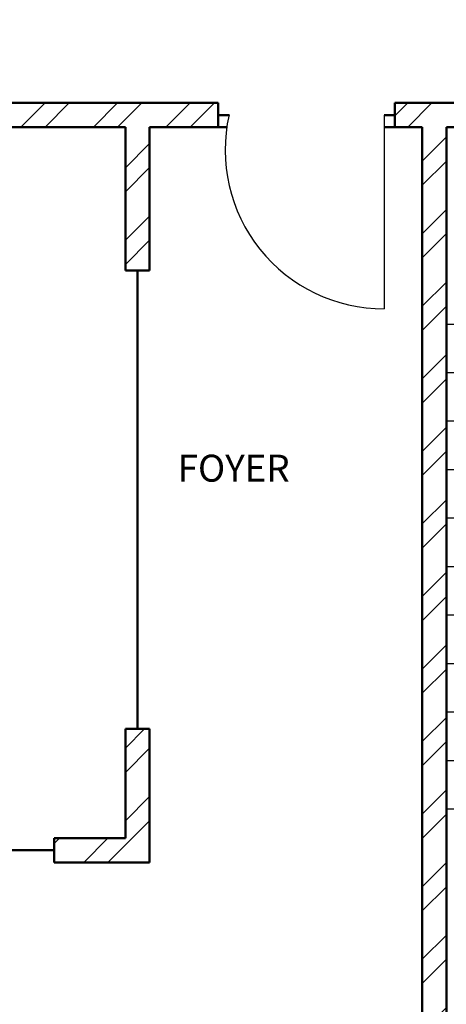
# Model space of a CAD drawing. Units: inches. Extents: x 1901 to 2863, y 888 to 2433.
# Tile 20 of 91: x 2264 to 2343, y 1549 to 1732. Entities that reach past the tile are written whole.
import ezdxf

# ---------------------------------------------------------------- set-up
doc = ezdxf.new("R2010")
doc.units = ezdxf.units.IN
for name, color, linetype, lineweight in [('A-AREA-IDEN', 7, 'Continuous', 18), ('A-DOOR', 4, 'Continuous', 25), ('A-FLOR-STRS', 2, 'Continuous', 25), ('A-WALL', 7, 'Continuous', 50), ('A-WALL-PATT', 8, 'Continuous', 13)]:
    doc.layers.add(name, color=color, linetype=linetype, lineweight=lineweight)
doc.styles.get("Standard").update_dxf_attribs({"font": 'arial.ttf'})

msp = doc.modelspace()

# ---------------------------------------------------------------- hatches: boundary and pattern name
at = {"layer": 'A-WALL-PATT'}
h = msp.add_hatch(dxfattribs=at)
h.set_pattern_fill('ANSI32', color=256)
h.paths.add_polyline_path([(2192.5, 2274.13), (2141.26, 2274.13), (2141.26, 2269.63), (2192.5, 2269.63)])
h.paths.add_polyline_path([(2259.93, 2274.13), (2216.5, 2274.13), (2216.5, 2269.63), (2255.43, 2269.63), (2255.43, 2214.63), (2250.81, 2214.63), (2250.81, 2210.13), (2259.93, 2210.13), (2259.93, 2215.13), (2271.76, 2215.13), (2271.76, 2217.38), (2271.76, 2219.63), (2259.93, 2219.63)])
h.paths.add_polyline_path([(2171.43, 2269.63), (2166.93, 2269.63), (2166.93, 2219.63), (2121.24, 2219.63), (2121.24, 2215.13), (2166.93, 2215.13), (2166.93, 2083.13), (2161.81, 2083.13), (2161.81, 2078.63), (2171.43, 2078.63), (2177, 2078.63), (2177, 2080.88), (2177, 2083.13), (2171.43, 2083.13), (2171.43, 2210.13), (2230.91, 2210.13), (2230.91, 2212.38), (2230.91, 2214.63), (2171.43, 2214.63)])
h.paths.add_polyline_path([(2117.26, 2274.13), (2089.43, 2274.13), (2089.43, 2219.63), (2081.14, 2219.63), (2081.14, 2215.13), (2089.43, 2215.13), (2098, 2215.13), (2098, 2217.38), (2098, 2219.63), (2093.93, 2219.63), (2093.93, 2269.63), (2117.26, 2269.63), (2117.26, 2271.88)])
h.paths.add_polyline_path([(2343.43, 2219.63), (2329.29, 2219.63), (2329.29, 2215.13), (2338.93, 2215.13), (2338.93, 2184.74), (2343.43, 2184.74)])
h.paths.add_polyline_path([(2338.93, 2083.13), (2329.29, 2083.13), (2208.97, 2083.13), (2208.97, 2078.63), (2338.93, 2078.63)])
h.paths.add_polyline_path([(2343.43, 2136.74), (2338.93, 2136.74), (2338.93, 1872.63), (2343.43, 1872.63)])
h.paths.add_polyline_path([(2343.43, 1863.63), (2397.68, 1863.63), (2397.68, 1821.63), (2384.14, 1821.63), (2384.14, 1812.63), (2418.33, 1812.63), (2418.33, 1817.13), (2418.33, 1821.63), (2406.68, 1821.63), (2406.68, 1863.63), (2459.5, 1863.63), (2459.5, 1821.63), (2447.14, 1821.63), (2447.14, 1812.63), (2459.5, 1812.63), (2468.5, 1812.63), (2468.5, 1872.63), (2394.43, 1872.63), (2334.43, 1872.63), (2334.43, 1812.63), (2343.43, 1812.63), (2353.25, 1812.63), (2353.25, 1821.63), (2343.43, 1821.63)])
h.paths.add_polyline_path([(2510.01, 1872.63), (2468.5, 1872.63), (2468.5, 1868.13), (2510.01, 1868.13)])
h.paths.add_polyline_path([(2514.01, 1817.13), (2468.5, 1817.13), (2468.5, 1812.63), (2482.11, 1812.63), (2482.11, 1800.61), (2486.61, 1800.61), (2486.61, 1812.63), (2514.01, 1812.63)])
h.paths.add_polyline_path([(2299.25, 1814.88), (2299.25, 1817.13), (2295.93, 1817.13), (2295.93, 1854.17), (2293.68, 1854.17), (2291.43, 1854.17), (2291.43, 1817.13), (2266.11, 1817.13), (2266.11, 1812.63), (2299.25, 1812.63)])
h.paths.add_polyline_path([(2218.11, 1817.13), (2206.46, 1817.13), (2171.43, 1817.13), (2171.43, 1949.13), (2190.1, 1949.13), (2190.1, 1953.63), (2163.47, 1953.63), (2163.47, 1949.13), (2166.93, 1949.13), (2166.93, 1817.13), (2114.3, 1817.13), (2114.3, 1812.63), (2218.11, 1812.63)])
h.paths.add_polyline_path([(2029.43, 1970.92), (2024.93, 1970.92), (2024.93, 1912.72), (2029.43, 1912.72)])
h.paths.add_polyline_path([(2132.3, 1953.63), (2113.93, 1953.63), (2113.93, 1975.89), (2111.68, 1975.89), (2109.43, 1975.89), (2109.43, 1953.63), (2029.43, 1953.63), (2029.43, 1949.13), (2132.3, 1949.13)])
h.paths.add_polyline_path([(2029.43, 1853.61), (2029.31, 1853.61), (2029.31, 1853.61), (2029.43, 1853.61), (2029.43, 1864.72), (2024.93, 1864.72), (2024.93, 1812.63), (2066.3, 1812.63), (2066.3, 1814.88), (2066.3, 1817.13), (2029.43, 1817.13)])
h.paths.add_polyline_path([(2122.93, 2010.09), (2120.68, 2010.09), (2118.43, 2010.09), (2118.43, 2006.13), (2029.43, 2006.13), (2029.43, 2001.63), (2109.43, 2001.63), (2109.43, 1998.04), (2113.93, 1998.04), (2113.93, 2001.63), (2122.93, 2001.63)])
h.paths.add_polyline_path([(2029.43, 2031.38), (2024.93, 2031.38), (2024.93, 1994.92), (2027.18, 1994.92), (2029.43, 1994.92)])
h.paths.add_polyline_path([(2029.43, 2136.74), (2024.93, 2136.74), (2024.93, 2067.38), (2027.18, 2067.38), (2029.43, 2067.38)])
h.paths.add_polyline_path([(2125.62, 2083.13), (2029.43, 2083.13), (2029.43, 2078.63), (2118.43, 2078.63), (2118.43, 2030.71), (2122.93, 2030.71), (2122.93, 2078.63), (2125.62, 2078.63)])
h.paths.add_polyline_path([(2029.43, 2215.13), (2040.47, 2215.13), (2040.47, 2217.38), (2040.47, 2219.63), (2024.93, 2219.63), (2024.93, 2184.74), (2029.43, 2184.74), (2029.43, 2187.78)])
h.paths.add_polyline_path([(2686.43, 2274.13), (2659.28, 2274.13), (2659.28, 2269.63), (2681.93, 2269.63), (2681.93, 2219.63), (2676.82, 2219.63), (2676.82, 2215.13), (2681.93, 2215.13), (2697.01, 2215.13), (2697.01, 2217.38), (2697.01, 2219.63), (2686.43, 2219.63)])
h.paths.add_polyline_path([(2609.93, 2269.63), (2635.28, 2269.63), (2635.28, 2274.13), (2571.43, 2274.13), (2571.43, 2269.63), (2605.43, 2269.63), (2605.43, 2214.63), (2549.1, 2214.63), (2549.1, 2210.13), (2605.43, 2210.13), (2605.43, 2083.13), (2601.01, 2083.13), (2601.01, 2080.88), (2601.01, 2078.63), (2609.93, 2078.63), (2616.16, 2078.63), (2616.16, 2080.88), (2616.16, 2083.13), (2609.93, 2083.13), (2609.93, 2215.13), (2651.46, 2215.13), (2651.46, 2217.38), (2651.46, 2219.63), (2609.93, 2219.63)])
h.paths.add_polyline_path([(2521.43, 2269.63), (2547.43, 2269.63), (2547.43, 2271.88), (2547.43, 2274.13), (2516.93, 2274.13), (2516.93, 2219.63), (2506.41, 2219.63), (2506.41, 2215.13), (2516.93, 2215.13), (2516.93, 2210.13), (2525.4, 2210.13), (2525.4, 2212.38), (2525.4, 2214.63), (2521.43, 2214.63)])
h.paths.add_polyline_path([(2456.01, 2219.63), (2439.43, 2219.63), (2439.43, 2187.89), (2443.93, 2187.89), (2443.93, 2215.13), (2456.01, 2215.13)])
h.paths.add_polyline_path([(2752.93, 2219.63), (2739.48, 2219.63), (2739.48, 2215.13), (2748.43, 2215.13), (2748.43, 2187.89), (2752.93, 2187.89)])
h.paths.add_polyline_path([(2752.93, 2139.89), (2748.43, 2139.89), (2748.43, 2083.13), (2648.42, 2083.13), (2648.42, 2078.63), (2654.93, 2078.63), (2654.93, 2039.44), (2659.43, 2039.44), (2659.43, 2078.63), (2748.43, 2078.63), (2748.43, 2063.43), (2752.93, 2063.43)])
h.paths.add_polyline_path([(2752.93, 2010.63), (2659.43, 2010.63), (2659.43, 2015.65), (2654.93, 2015.65), (2654.93, 2010.63), (2605.43, 2010.63), (2605.43, 1920.97), (2609.93, 1920.97), (2609.93, 2006.13), (2748.43, 2006.13), (2748.43, 1982.47), (2752.93, 1982.47)])
h.paths.add_polyline_path([(2752.93, 2027.43), (2748.43, 2027.43), (2748.43, 2010.63), (2752.93, 2010.63)])
h.paths.add_polyline_path([(2748.43, 1886.13), (2609.93, 1886.13), (2609.93, 1889.72), (2605.43, 1889.72), (2605.43, 1861.26), (2609.93, 1861.26), (2609.93, 1881.63), (2748.43, 1881.63)])
h.paths.add_polyline_path([(2456.86, 2228.83), (2498.4, 2228.83), (2498.4, 2247.49), (2456.86, 2247.49)], flags=9)
h.paths.add_polyline_path([(2038.6, 2237.42), (2080.17, 2237.42), (2080.17, 2256.08), (2038.6, 2256.08)], flags=9)
h.paths.add_polyline_path([(2292.01, 1062.39), (2539.93, 1062.39), (2539.93, 1099.49), (2292.01, 1099.49)], flags=9)
h.paths.add_polyline_path([(2424.91, 1832.25), (2448.51, 1832.25), (2448.51, 1846.68), (2424.91, 1846.68)], flags=25)
h.paths.add_polyline_path([(2359.08, 1832.25), (2382.68, 1832.25), (2382.68, 1846.68), (2359.08, 1846.68)], flags=25)
h.paths.add_polyline_path([(2352.9, 1684.8), (2367.54, 1684.8), (2367.54, 1697.17), (2352.9, 1697.17)], flags=9)
h.paths.add_polyline_path([(2079.29, 1755.83), (2169.02, 1755.83), (2169.02, 1774.37), (2079.29, 1774.37)], flags=9)
h.paths.add_polyline_path([(2404.09, 1373.86), (2404.09, 1463.59), (2385.54, 1463.59), (2385.54, 1373.86)], flags=9)
h.paths.add_polyline_path([(2268.09, 2236.37), (2309.64, 2236.37), (2309.64, 2255.03), (2268.09, 2255.03)], flags=9)
h.paths.add_polyline_path([(2575.96, 1700.95), (2665.7, 1700.95), (2665.7, 1719.5), (2575.96, 1719.5)], flags=9)
h.paths.add_polyline_path([(2302.96, 1878.47), (2329.52, 1878.47), (2329.52, 1888.78), (2302.96, 1888.78)], flags=9)
h.paths.add_polyline_path([(2097.42, 2240.58), (2126.57, 2240.58), (2126.57, 2259.23), (2097.42, 2259.23)], flags=9)
h.paths.add_polyline_path([(2208.72, 2246.12), (2237.88, 2246.12), (2237.88, 2264.78), (2208.72, 2264.78)], flags=9)
h.paths.add_polyline_path([(2038.15, 1925.96), (2076.99, 1925.96), (2076.99, 1944.62), (2038.15, 1944.62)], flags=9)
h.paths.add_polyline_path([(2239.14, 1926.67), (2288.46, 1926.67), (2288.46, 1945.33), (2239.14, 1945.33)], flags=9)
h.paths.add_polyline_path([(2175.43, 2007.33), (2212.36, 2007.33), (2212.36, 2025.99), (2175.43, 2025.99)], flags=9)
h.paths.add_polyline_path([(2225.03, 2091.79), (2263.87, 2091.79), (2263.87, 2110.45), (2225.03, 2110.45)], flags=9)
h.paths.add_polyline_path([(2035.4, 2098.48), (2074.24, 2098.48), (2074.24, 2117.14), (2035.4, 2117.14)], flags=9)
h.paths.add_polyline_path([(2050.1, 2029.21), (2083.26, 2029.21), (2083.26, 2047.87), (2050.1, 2047.87)], flags=9)
h.paths.add_polyline_path([(2069.68, 1956.72), (2098.83, 1956.72), (2098.83, 1975.38), (2069.68, 1975.38)], flags=25)
h.paths.add_polyline_path([(2328.62, 1753.34), (2361.66, 1753.34), (2361.66, 1771.99), (2328.62, 1771.99)], flags=9)
h.paths.add_polyline_path([(2395.16, 2060.89), (2395.16, 2140.65), (2378.68, 2140.65), (2378.68, 2060.89)], flags=9)
h.paths.add_polyline_path([(2463.73, 2059.02), (2492.89, 2059.02), (2492.89, 2077.68), (2463.73, 2077.68)], flags=9)
h.paths.add_polyline_path([(2458.03, 2181.54), (2496.87, 2181.54), (2496.87, 2200.19), (2458.03, 2200.19)], flags=9)
h.paths.add_polyline_path([(2527.58, 2243.07), (2556.73, 2243.07), (2556.73, 2261.73), (2527.58, 2261.73)], flags=9)
h.paths.add_polyline_path([(2694.46, 2232.77), (2736.03, 2232.77), (2736.03, 2251.42), (2694.46, 2251.42)], flags=9)
h.paths.add_polyline_path([(2637.82, 2249.22), (2666.98, 2249.22), (2666.98, 2267.88), (2637.82, 2267.88)], flags=9)
h.paths.add_polyline_path([(2623.69, 2183.54), (2662.53, 2183.54), (2662.53, 2202.2), (2623.69, 2202.2)], flags=9)
h.paths.add_polyline_path([(2691.97, 2021.5), (2725.12, 2021.5), (2725.12, 2040.16), (2691.97, 2040.16)], flags=9)
h.paths.add_polyline_path([(2621.04, 1975.91), (2662.34, 1975.91), (2662.34, 1994.57), (2621.04, 1994.57)], flags=25)
h.paths.add_polyline_path([(2479.03, 1927.62), (2519.84, 1927.62), (2519.84, 1946.28), (2479.03, 1946.28)], flags=9)
h.paths.add_polyline_path([(2670.94, 1849.08), (2716.01, 1849.08), (2716.01, 1867.73), (2670.94, 1867.73)], flags=9)
h.paths.add_polyline_path([(2523.61, 1782.96), (2550.17, 1782.96), (2550.17, 1793.26), (2523.61, 1793.26)], flags=9)
h.paths.add_polyline_path([(2450.84, 1207.33), (2492.39, 1207.33), (2492.39, 1225.99), (2450.84, 1225.99)], flags=9)
h.paths.add_polyline_path([(2527.75, 1203.84), (2556.91, 1203.84), (2556.91, 1222.5), (2527.75, 1222.5)], flags=9)
h.paths.add_polyline_path([(2639.11, 1207.2), (2668.27, 1207.2), (2668.27, 1225.86), (2639.11, 1225.86)], flags=9)
h.paths.add_polyline_path([(2692.59, 1218.97), (2734.17, 1218.97), (2734.17, 1237.62), (2692.59, 1237.62)], flags=9)
h.paths.add_polyline_path([(2669.27, 1366.33), (2708.11, 1366.33), (2708.11, 1384.99), (2669.27, 1384.99)], flags=9)
h.paths.add_polyline_path([(2463.31, 1358.03), (2502.15, 1358.03), (2502.15, 1376.69), (2463.31, 1376.69)], flags=9)
h.paths.add_polyline_path([(2494.72, 1449.96), (2531.65, 1449.96), (2531.65, 1468.62), (2494.72, 1468.62)], flags=9)
h.paths.add_polyline_path([(2675.57, 1422.16), (2708.72, 1422.16), (2708.72, 1440.81), (2675.57, 1440.81)], flags=9)
h.paths.add_polyline_path([(2685.63, 1493.89), (2714.79, 1493.89), (2714.79, 1512.55), (2685.63, 1512.55)], flags=9)
h.paths.add_polyline_path([(2686.8, 1529.91), (2725.65, 1529.91), (2725.65, 1548.57), (2686.8, 1548.57)], flags=9)
h.paths.add_polyline_path([(2503.65, 1537.99), (2552.97, 1537.99), (2552.97, 1556.65), (2503.65, 1556.65)], flags=9)
h.paths.add_polyline_path([(2291.71, 1643.5), (2318.28, 1643.5), (2318.28, 1653.81), (2291.71, 1653.81)], flags=9)
h.paths.add_polyline_path([(2450.63, 1610.52), (2477.19, 1610.52), (2477.19, 1620.82), (2450.63, 1620.82)], flags=9)
h.paths.add_polyline_path([(2359.99, 1551.81), (2422.25, 1551.81), (2422.25, 1562.12), (2359.99, 1562.12)], flags=9)
h.paths.add_polyline_path([(2280.11, 1249.01), (2321.65, 1249.01), (2321.65, 1267.66), (2280.11, 1267.66)], flags=9)
h.paths.add_polyline_path([(2164.06, 1274.23), (2193.22, 1274.23), (2193.22, 1292.89), (2164.06, 1292.89)], flags=9)
h.paths.add_polyline_path([(2118.21, 1277.69), (2151.25, 1277.69), (2151.25, 1296.35), (2118.21, 1296.35)], flags=9)
h.paths.add_polyline_path([(2031.95, 1268.53), (2073.52, 1268.53), (2073.52, 1287.19), (2031.95, 1287.19)], flags=9)
h.paths.add_polyline_path([(2050.2, 1409.08), (2089.04, 1409.08), (2089.04, 1427.74), (2050.2, 1427.74)], flags=9)
h.paths.add_polyline_path([(2243.74, 1421.03), (2282.58, 1421.03), (2282.58, 1439.69), (2243.74, 1439.69)], flags=9)
h.paths.add_polyline_path([(2190.75, 1509.77), (2231.56, 1509.77), (2231.56, 1528.43), (2190.75, 1528.43)], flags=9)
h.paths.add_polyline_path([(2058.39, 1475.42), (2091.55, 1475.42), (2091.55, 1494.07), (2058.39, 1494.07)], flags=9)
h.paths.add_polyline_path([(2062.45, 1553.09), (2091.6, 1553.09), (2091.6, 1571.75), (2062.45, 1571.75)], flags=9)
h.paths.add_polyline_path([(2219.52, 1590.37), (2266.15, 1590.37), (2266.15, 1609.02), (2219.52, 1609.02)], flags=9)
h.paths.add_polyline_path([(2041.07, 1584.19), (2079.91, 1584.19), (2079.91, 1602.85), (2041.07, 1602.85)], flags=9)
h = msp.add_hatch(dxfattribs=at)
h.set_pattern_fill('ANSI32', color=256)
h.paths.add_polyline_path([(2443.93, 2139.89), (2439.43, 2139.89), (2439.43, 2069.35), (2441.68, 2069.35), (2443.93, 2069.35), (2443.93, 2078.63), (2521.93, 2078.63), (2521.93, 2075.07), (2524.18, 2075.07), (2526.43, 2075.07), (2526.43, 2078.63), (2571.75, 2078.63), (2571.75, 2080.88), (2571.75, 2083.13), (2443.93, 2083.13)])
h.paths.add_polyline_path([(2526.43, 2054.63), (2524.18, 2054.63), (2521.93, 2054.63), (2521.93, 2030.63), (2443.93, 2030.63), (2443.93, 2045.35), (2439.43, 2045.35), (2439.43, 1983.87), (2443.93, 1983.87), (2443.93, 2026.13), (2521.93, 2026.13), (2526.43, 2026.13)])
h.paths.add_polyline_path([(2443.93, 1923.87), (2439.43, 1923.87), (2439.43, 1872.63), (2443.93, 1872.63)])
h.paths.add_polyline_path([(2636.23, 1766.13), (2609.93, 1766.13), (2609.93, 1779.79), (2605.43, 1779.79), (2605.43, 1766.13), (2486.61, 1766.13), (2486.61, 1770.67), (2482.11, 1770.67), (2482.11, 1766.13), (2482.11, 1761.63), (2636.23, 1761.63), (2636.23, 1763.88)])
h.paths.add_polyline_path([(2519.54, 1663.38), (2519.54, 1665.63), (2494.93, 1665.63), (2481.83, 1665.63), (2481.83, 1663.38), (2481.83, 1661.13), (2490.43, 1661.13), (2490.43, 1640.16), (2494.93, 1640.16), (2494.93, 1661.13), (2519.54, 1661.13)])
h.paths.add_polyline_path([(2443.93, 1712.13), (2443.93, 1716.63), (2414.46, 1716.63), (2414.46, 1712.13), (2439.43, 1712.13), (2439.43, 1545.51), (2443.93, 1545.51), (2443.93, 1661.13), (2448.47, 1661.13), (2448.47, 1665.63), (2443.93, 1665.63)])
h.paths.add_polyline_path([(2343.43, 1712.13), (2365.52, 1712.13), (2365.52, 1714.38), (2365.52, 1716.63), (2333.87, 1716.63), (2333.87, 1714.38), (2333.87, 1712.13), (2338.93, 1712.13), (2338.93, 1575.63), (2338.93, 1545.51), (2343.43, 1545.51), (2343.43, 1547.51), (2343.43, 1580.13)])
h.paths.add_polyline_path([(2752.93, 1665.63), (2579.54, 1665.63), (2579.54, 1661.13), (2615.93, 1661.13), (2615.93, 1529.13), (2598.93, 1529.13), (2598.93, 1524.63), (2623.13, 1524.63), (2623.13, 1526.88), (2623.13, 1529.13), (2620.43, 1529.13), (2620.43, 1661.13), (2748.43, 1661.13), (2748.43, 1633.5), (2752.93, 1633.5)])
h.paths.add_polyline_path([(2752.93, 1419.93), (2748.43, 1419.93), (2748.43, 1400.13), (2659.43, 1400.13), (2659.43, 1444.33), (2657.18, 1444.33), (2654.93, 1444.33), (2654.93, 1400.13), (2643.65, 1400.13), (2643.65, 1395.63), (2748.43, 1395.63), (2748.43, 1364.04), (2752.93, 1364.04)])
h.paths.add_polyline_path([(2752.93, 1492.88), (2748.43, 1492.88), (2748.43, 1476.63), (2667.43, 1476.63), (2667.43, 1479.71), (2665.18, 1479.71), (2662.93, 1479.71), (2662.93, 1476.63), (2654.93, 1476.63), (2654.93, 1469.54), (2659.43, 1469.54), (2659.43, 1472.13), (2748.43, 1472.13), (2748.43, 1455.93), (2752.93, 1455.93)])
h.paths.add_polyline_path([(2752.93, 1304.04), (2748.43, 1304.04), (2748.43, 1263.63), (2738.66, 1263.63), (2738.66, 1259.13), (2752.93, 1259.13)])
h.paths.add_polyline_path([(2685.93, 1259.13), (2695.49, 1259.13), (2695.49, 1261.38), (2695.49, 1263.63), (2677.84, 1263.63), (2677.84, 1261.38), (2677.84, 1259.13), (2681.43, 1259.13), (2681.43, 1203.63), (2653.28, 1203.63), (2653.28, 1199.13), (2685.93, 1199.13), (2685.93, 1203.63)])
h.paths.add_polyline_path([(2609.43, 1395.63), (2611.85, 1395.63), (2611.85, 1400.13), (2598.89, 1400.13), (2598.89, 1397.88), (2598.89, 1395.63), (2604.93, 1395.63), (2604.93, 1268.13), (2554.73, 1268.13), (2554.73, 1265.88), (2554.73, 1263.63), (2604.93, 1263.63), (2604.93, 1203.63), (2571.31, 1203.63), (2571.31, 1199.13), (2604.93, 1199.13), (2629.28, 1199.13), (2629.28, 1201.38), (2629.28, 1203.63), (2609.43, 1203.63), (2609.43, 1258.63), (2609.43, 1259.13), (2654.8, 1259.13), (2654.8, 1263.63), (2609.43, 1263.63)])
h.paths.add_polyline_path([(2443.93, 1304.04), (2439.43, 1304.04), (2439.43, 1259.13), (2443.93, 1259.13), (2456.16, 1259.13), (2456.16, 1261.38), (2456.16, 1263.63), (2443.93, 1263.63)])
h.paths.add_polyline_path([(2525.43, 1263.63), (2531.78, 1263.63), (2531.78, 1268.13), (2520.93, 1268.13), (2520.93, 1263.63), (2511.41, 1263.63), (2511.41, 1259.13), (2520.93, 1259.13), (2520.93, 1199.13), (2547.31, 1199.13), (2547.31, 1201.38), (2547.31, 1203.63), (2525.43, 1203.63)])
h.paths.add_polyline_path([(2443.93, 1434.84), (2439.43, 1434.84), (2439.43, 1364.04), (2441.68, 1364.04), (2443.93, 1364.04)])
h.paths.add_polyline_path([(2567.13, 1400.13), (2443.93, 1400.13), (2443.93, 1395.63), (2567.13, 1395.63)])
h.paths.add_polyline_path([(2443.93, 1545.51), (2439.43, 1545.51), (2439.43, 1494.84), (2443.93, 1494.84)])
h.paths.add_polyline_path([(2494.93, 1553.35), (2492.68, 1553.35), (2490.43, 1553.35), (2490.43, 1524.63), (2494.93, 1524.63), (2525.94, 1524.63), (2525.94, 1526.88), (2525.94, 1529.13), (2494.93, 1529.13)])
h.paths.add_polyline_path([(2752.93, 1573.5), (2748.43, 1573.5), (2748.43, 1529.13), (2657.76, 1529.13), (2657.76, 1524.63), (2662.93, 1524.63), (2662.93, 1498.63), (2667.43, 1498.63), (2667.43, 1524.63), (2748.43, 1524.63), (2748.43, 1516.88), (2752.93, 1516.88)])
h.paths.add_polyline_path([(2038.6, 2237.42), (2080.17, 2237.42), (2080.17, 2256.08), (2038.6, 2256.08)], flags=9)
h.paths.add_polyline_path([(2292.01, 1062.39), (2539.93, 1062.39), (2539.93, 1099.49), (2292.01, 1099.49)], flags=9)
h.paths.add_polyline_path([(2424.91, 1832.25), (2448.51, 1832.25), (2448.51, 1846.68), (2424.91, 1846.68)], flags=9)
h.paths.add_polyline_path([(2359.08, 1832.25), (2382.68, 1832.25), (2382.68, 1846.68), (2359.08, 1846.68)], flags=9)
h.paths.add_polyline_path([(2352.9, 1684.8), (2367.54, 1684.8), (2367.54, 1697.17), (2352.9, 1697.17)], flags=9)
h.paths.add_polyline_path([(2079.29, 1755.83), (2169.02, 1755.83), (2169.02, 1774.37), (2079.29, 1774.37)], flags=9)
h.paths.add_polyline_path([(2404.09, 1373.86), (2404.09, 1463.59), (2385.54, 1463.59), (2385.54, 1373.86)], flags=9)
h.paths.add_polyline_path([(2268.09, 2236.37), (2309.64, 2236.37), (2309.64, 2255.03), (2268.09, 2255.03)], flags=9)
h.paths.add_polyline_path([(2575.96, 1700.95), (2665.7, 1700.95), (2665.7, 1719.5), (2575.96, 1719.5)], flags=9)
h.paths.add_polyline_path([(2302.96, 1878.47), (2329.52, 1878.47), (2329.52, 1888.78), (2302.96, 1888.78)], flags=9)
h.paths.add_polyline_path([(2097.42, 2240.58), (2126.57, 2240.58), (2126.57, 2259.23), (2097.42, 2259.23)], flags=9)
h.paths.add_polyline_path([(2208.72, 2246.12), (2237.88, 2246.12), (2237.88, 2264.78), (2208.72, 2264.78)], flags=9)
h.paths.add_polyline_path([(2038.15, 1925.96), (2076.99, 1925.96), (2076.99, 1944.62), (2038.15, 1944.62)], flags=9)
h.paths.add_polyline_path([(2239.14, 1926.67), (2288.46, 1926.67), (2288.46, 1945.33), (2239.14, 1945.33)], flags=9)
h.paths.add_polyline_path([(2175.43, 2007.33), (2212.36, 2007.33), (2212.36, 2025.99), (2175.43, 2025.99)], flags=9)
h.paths.add_polyline_path([(2225.03, 2091.79), (2263.87, 2091.79), (2263.87, 2110.45), (2225.03, 2110.45)], flags=9)
h.paths.add_polyline_path([(2035.4, 2098.48), (2074.24, 2098.48), (2074.24, 2117.14), (2035.4, 2117.14)], flags=9)
h.paths.add_polyline_path([(2050.1, 2029.21), (2083.26, 2029.21), (2083.26, 2047.87), (2050.1, 2047.87)], flags=9)
h.paths.add_polyline_path([(2069.68, 1956.72), (2098.83, 1956.72), (2098.83, 1975.38), (2069.68, 1975.38)], flags=9)
h.paths.add_polyline_path([(2328.62, 1753.34), (2361.66, 1753.34), (2361.66, 1771.99), (2328.62, 1771.99)], flags=9)
h.paths.add_polyline_path([(2395.16, 2060.89), (2395.16, 2140.65), (2378.68, 2140.65), (2378.68, 2060.89)], flags=9)
h.paths.add_polyline_path([(2463.73, 2059.02), (2492.89, 2059.02), (2492.89, 2077.68), (2463.73, 2077.68)], flags=9)
h.paths.add_polyline_path([(2458.03, 2181.54), (2496.87, 2181.54), (2496.87, 2200.19), (2458.03, 2200.19)], flags=9)
h.paths.add_polyline_path([(2456.86, 2228.83), (2498.4, 2228.83), (2498.4, 2247.49), (2456.86, 2247.49)], flags=9)
h.paths.add_polyline_path([(2527.58, 2243.07), (2556.73, 2243.07), (2556.73, 2261.73), (2527.58, 2261.73)], flags=9)
h.paths.add_polyline_path([(2694.46, 2232.77), (2736.03, 2232.77), (2736.03, 2251.42), (2694.46, 2251.42)], flags=9)
h.paths.add_polyline_path([(2637.82, 2249.22), (2666.98, 2249.22), (2666.98, 2267.88), (2637.82, 2267.88)], flags=9)
h.paths.add_polyline_path([(2623.69, 2183.54), (2662.53, 2183.54), (2662.53, 2202.2), (2623.69, 2202.2)], flags=9)
h.paths.add_polyline_path([(2691.97, 2021.5), (2725.12, 2021.5), (2725.12, 2040.16), (2691.97, 2040.16)], flags=9)
h.paths.add_polyline_path([(2621.04, 1975.91), (2662.34, 1975.91), (2662.34, 1994.57), (2621.04, 1994.57)], flags=9)
h.paths.add_polyline_path([(2479.03, 1927.62), (2519.84, 1927.62), (2519.84, 1946.28), (2479.03, 1946.28)], flags=9)
h.paths.add_polyline_path([(2670.94, 1849.08), (2716.01, 1849.08), (2716.01, 1867.73), (2670.94, 1867.73)], flags=9)
h.paths.add_polyline_path([(2523.61, 1782.96), (2550.17, 1782.96), (2550.17, 1793.26), (2523.61, 1793.26)], flags=9)
h.paths.add_polyline_path([(2450.84, 1207.33), (2492.39, 1207.33), (2492.39, 1225.99), (2450.84, 1225.99)], flags=9)
h.paths.add_polyline_path([(2527.75, 1203.84), (2556.91, 1203.84), (2556.91, 1222.5), (2527.75, 1222.5)], flags=9)
h.paths.add_polyline_path([(2639.11, 1207.2), (2668.27, 1207.2), (2668.27, 1225.86), (2639.11, 1225.86)], flags=9)
h.paths.add_polyline_path([(2692.59, 1218.97), (2734.17, 1218.97), (2734.17, 1237.62), (2692.59, 1237.62)], flags=9)
h.paths.add_polyline_path([(2669.27, 1366.33), (2708.11, 1366.33), (2708.11, 1384.99), (2669.27, 1384.99)], flags=25)
h.paths.add_polyline_path([(2463.31, 1358.03), (2502.15, 1358.03), (2502.15, 1376.69), (2463.31, 1376.69)], flags=9)
h.paths.add_polyline_path([(2494.72, 1449.96), (2531.65, 1449.96), (2531.65, 1468.62), (2494.72, 1468.62)], flags=9)
h.paths.add_polyline_path([(2675.57, 1422.16), (2708.72, 1422.16), (2708.72, 1440.81), (2675.57, 1440.81)], flags=25)
h.paths.add_polyline_path([(2685.63, 1493.89), (2714.79, 1493.89), (2714.79, 1512.55), (2685.63, 1512.55)], flags=9)
h.paths.add_polyline_path([(2686.8, 1529.91), (2725.65, 1529.91), (2725.65, 1548.57), (2686.8, 1548.57)], flags=25)
h.paths.add_polyline_path([(2503.65, 1537.99), (2552.97, 1537.99), (2552.97, 1556.65), (2503.65, 1556.65)], flags=9)
h.paths.add_polyline_path([(2291.71, 1643.5), (2318.28, 1643.5), (2318.28, 1653.81), (2291.71, 1653.81)], flags=9)
h.paths.add_polyline_path([(2450.63, 1610.52), (2477.19, 1610.52), (2477.19, 1620.82), (2450.63, 1620.82)], flags=9)
h.paths.add_polyline_path([(2359.99, 1551.81), (2422.25, 1551.81), (2422.25, 1562.12), (2359.99, 1562.12)], flags=9)
h.paths.add_polyline_path([(2280.11, 1249.01), (2321.65, 1249.01), (2321.65, 1267.66), (2280.11, 1267.66)], flags=9)
h.paths.add_polyline_path([(2164.06, 1274.23), (2193.22, 1274.23), (2193.22, 1292.89), (2164.06, 1292.89)], flags=9)
h.paths.add_polyline_path([(2118.21, 1277.69), (2151.25, 1277.69), (2151.25, 1296.35), (2118.21, 1296.35)], flags=9)
h.paths.add_polyline_path([(2031.95, 1268.53), (2073.52, 1268.53), (2073.52, 1287.19), (2031.95, 1287.19)], flags=9)
h.paths.add_polyline_path([(2050.2, 1409.08), (2089.04, 1409.08), (2089.04, 1427.74), (2050.2, 1427.74)], flags=9)
h.paths.add_polyline_path([(2243.74, 1421.03), (2282.58, 1421.03), (2282.58, 1439.69), (2243.74, 1439.69)], flags=9)
h.paths.add_polyline_path([(2190.75, 1509.77), (2231.56, 1509.77), (2231.56, 1528.43), (2190.75, 1528.43)], flags=9)
h.paths.add_polyline_path([(2058.39, 1475.42), (2091.55, 1475.42), (2091.55, 1494.07), (2058.39, 1494.07)], flags=9)
h.paths.add_polyline_path([(2062.45, 1553.09), (2091.6, 1553.09), (2091.6, 1571.75), (2062.45, 1571.75)], flags=9)
h.paths.add_polyline_path([(2219.52, 1590.37), (2266.15, 1590.37), (2266.15, 1609.02), (2219.52, 1609.02)], flags=9)
h.paths.add_polyline_path([(2041.07, 1584.19), (2079.91, 1584.19), (2079.91, 1602.85), (2041.07, 1602.85)], flags=9)
h = msp.add_hatch(dxfattribs=at)
h.set_pattern_fill('ANSI32', color=256)
h.paths.add_polyline_path([(2182.93, 1716.63), (2024.93, 1716.63), (2024.93, 1681.7), (2029.33, 1681.7), (2029.33, 1712.13), (2154.33, 1712.13), (2154.33, 1580.13), (2148.52, 1580.13), (2148.52, 1577.88), (2148.52, 1575.63), (2194.93, 1575.63), (2194.93, 1580.13), (2158.83, 1580.13), (2158.83, 1712.13), (2182.93, 1712.13)])
h.paths.add_polyline_path([(2301.07, 1716.63), (2242.93, 1716.63), (2242.93, 1712.13), (2283.83, 1712.13), (2283.83, 1685.54), (2288.33, 1685.54), (2288.33, 1712.13), (2301.07, 1712.13)])
h.paths.add_polyline_path([(2288.33, 1600.41), (2286.08, 1600.41), (2283.83, 1600.41), (2283.83, 1580.13), (2270.6, 1580.13), (2270.6, 1575.63), (2288.33, 1575.63)])
h.paths.add_polyline_path([(2295.93, 1953.63), (2271.45, 1953.63), (2271.45, 1949.13), (2291.43, 1949.13), (2291.43, 1941.24), (2295.93, 1941.24)])
h.paths.add_polyline_path([(2098.38, 1244.13), (2082.33, 1244.13), (2082.33, 1302.13), (2086.52, 1302.13), (2086.52, 1306.63), (2067.46, 1306.63), (2067.46, 1302.13), (2077.83, 1302.13), (2077.83, 1239.63), (2098.38, 1239.63), (2098.38, 1241.88)])
h.paths.add_polyline_path([(2217.31, 1306.63), (2158.83, 1306.63), (2158.83, 1451.63), (2162.72, 1451.63), (2162.72, 1453.88), (2162.72, 1456.13), (2154.33, 1456.13), (2154.33, 1443.13), (2151.91, 1443.13), (2151.91, 1438.63), (2154.33, 1438.63), (2154.33, 1306.63), (2109.31, 1306.63), (2109.31, 1304.38), (2109.31, 1302.13), (2154.33, 1302.13), (2154.33, 1244.13), (2122.38, 1244.13), (2122.38, 1239.63), (2154.33, 1239.63), (2154.33, 1223.63), (2163.33, 1223.63), (2181.01, 1223.63), (2181.01, 1225.88), (2181.01, 1228.13), (2163.33, 1228.13), (2163.33, 1258.22), (2158.83, 1258.22), (2158.83, 1302.13), (2217.31, 1302.13)])
h.paths.add_polyline_path([(2259.99, 1306.63), (2238.3, 1306.63), (2238.3, 1304.38), (2238.3, 1302.13), (2242.83, 1302.13), (2242.83, 1228.13), (2205.01, 1228.13), (2205.01, 1223.63), (2247.33, 1223.63), (2247.33, 1302.13), (2259.99, 1302.13), (2259.99, 1304.38)])
h.paths.add_polyline_path([(2343.43, 1361.7), (2338.93, 1361.7), (2338.93, 1306.63), (2322.38, 1306.63), (2322.38, 1302.13), (2343.43, 1302.13)])
h.paths.add_polyline_path([(2343.43, 1470.4), (2338.93, 1470.4), (2338.93, 1456.13), (2193.73, 1456.13), (2193.73, 1453.88), (2193.73, 1451.63), (2338.93, 1451.63), (2338.93, 1421.7), (2343.43, 1421.7)])
h.paths.add_polyline_path([(2343.43, 1545.51), (2338.93, 1545.51), (2338.93, 1530.4), (2343.43, 1530.4)])
h.paths.add_polyline_path([(2029.33, 1466.83), (2024.93, 1466.83), (2024.93, 1409.82), (2029.33, 1409.82)])
h.paths.add_polyline_path([(2122.84, 1440.88), (2122.84, 1443.13), (2121.83, 1443.13), (2121.83, 1498.18), (2119.58, 1498.18), (2117.33, 1498.18), (2117.33, 1443.13), (2029.33, 1443.13), (2029.33, 1438.63), (2122.84, 1438.63)])
h.paths.add_polyline_path([(2029.33, 1543.05), (2024.93, 1543.05), (2024.93, 1502.83), (2029.33, 1502.83)])
h.paths.add_polyline_path([(2029.33, 1621.7), (2024.93, 1621.7), (2024.93, 1567.05), (2027.13, 1567.05), (2029.33, 1567.05), (2029.33, 1575.63), (2109.33, 1575.63), (2109.33, 1554.71), (2113.83, 1554.71), (2113.83, 1575.63), (2115.8, 1575.63), (2115.8, 1577.88), (2115.8, 1580.13), (2029.33, 1580.13)])
h.paths.add_polyline_path([(2121.83, 1527.63), (2117.33, 1527.63), (2113.83, 1527.63), (2113.83, 1533.01), (2111.58, 1533.01), (2109.33, 1533.01), (2109.33, 1527.63), (2029.33, 1527.63), (2029.33, 1523.13), (2117.33, 1523.13), (2117.33, 1519.43), (2121.83, 1519.43)])
h.paths.add_polyline_path([(2029.33, 1349.82), (2024.93, 1349.82), (2024.93, 1302.13), (2036.28, 1302.13), (2036.28, 1306.63), (2029.33, 1306.63)])

# ---------------------------------------------------------------- linework, layer by layer
at = {"layer": 'A-DOOR'}
msp.add_line((2331.87, 1714.38), (2331.87, 1678.38), dxfattribs=at)
msp.add_arc((2331.87, 1707.91), 29.52, 167.3246, 270, dxfattribs=at)
at = {"layer": 'A-FLOR-STRS'}
for p, q in [((2343.43, 1675.58), (2439.43, 1675.58)), ((2343.43, 1666.58), (2439.43, 1666.58)), ((2343.43, 1657.58), (2439.43, 1657.58)), ((2343.43, 1648.58), (2439.43, 1648.58)), ((2343.43, 1639.58), (2439.43, 1639.58)), ((2343.43, 1630.58), (2439.43, 1630.58)), ((2343.43, 1621.58), (2439.43, 1621.58)), ((2343.43, 1612.58), (2439.43, 1612.58)), ((2343.43, 1603.58), (2439.43, 1603.58)), ((2343.43, 1594.58), (2439.43, 1594.58)), ((2343.43, 1585.58), (2439.43, 1585.58))]:
    msp.add_line(p, q, dxfattribs=at)
at = {"layer": 'A-WALL'}
for p, q in [((2024.93, 1716.63), (2301.07, 1716.63)), ((2301.07, 1712.13), (2301.07, 1716.63)), ((2301.07, 1716.63), (2301.07, 1714.38)), ((2333.87, 1712.13), (2333.87, 1716.63)), ((2333.87, 1716.63), (2333.87, 1714.38)), ((2333.87, 1716.63), (2365.52, 1716.63)), ((2301.07, 1714.38), (2303.07, 1714.38)), ((2333.87, 1714.38), (2331.87, 1714.38)), ((2283.83, 1712.13), (2158.83, 1712.13)), ((2283.83, 1712.13), (2283.83, 1685.54)), ((2288.33, 1712.13), (2288.33, 1685.54)), ((2302.65, 1712.13), (2288.33, 1712.13)), ((2338.93, 1712.13), (2331.87, 1712.13)), ((2338.93, 1712.13), (2338.93, 1575.63)), ((2343.43, 1712.13), (2343.43, 1580.13)), ((2367.52, 1712.13), (2343.43, 1712.13)), ((2286.08, 1685.54), (2283.83, 1685.54)), ((2283.83, 1685.54), (2288.33, 1685.54)), ((2286.08, 1600.41), (2286.08, 1685.54)), ((2283.83, 1600.41), (2288.33, 1600.41)), ((2283.83, 1600.41), (2283.83, 1580.13)), ((2288.33, 1600.41), (2286.08, 1600.41)), ((2288.33, 1600.41), (2288.33, 1575.63)), ((2283.83, 1580.13), (2270.6, 1580.13)), ((2270.6, 1580.13), (2270.6, 1575.63)), ((2343.43, 1302.13), (2343.43, 1580.13)), ((2270.6, 1577.88), (2194.93, 1577.88)), ((2270.6, 1575.63), (2270.6, 1577.88)), ((2288.33, 1575.63), (2270.6, 1575.63)), ((2338.93, 1575.63), (2338.93, 1456.13))]:
    msp.add_line(p, q, dxfattribs=at)

# ---------------------------------------------------------------- texts
at = {"layer": 'A-AREA-IDEN', "insert": (2293.54, 1651.32), "char_height": 5, "attachment_point": 1}
msp.add_mtext_dynamic_manual_height_columns('FOYER', width=176.5358, gutter_width=12.5, heights=[0], dxfattribs=at)

doc.saveas('drawing.dxf')
